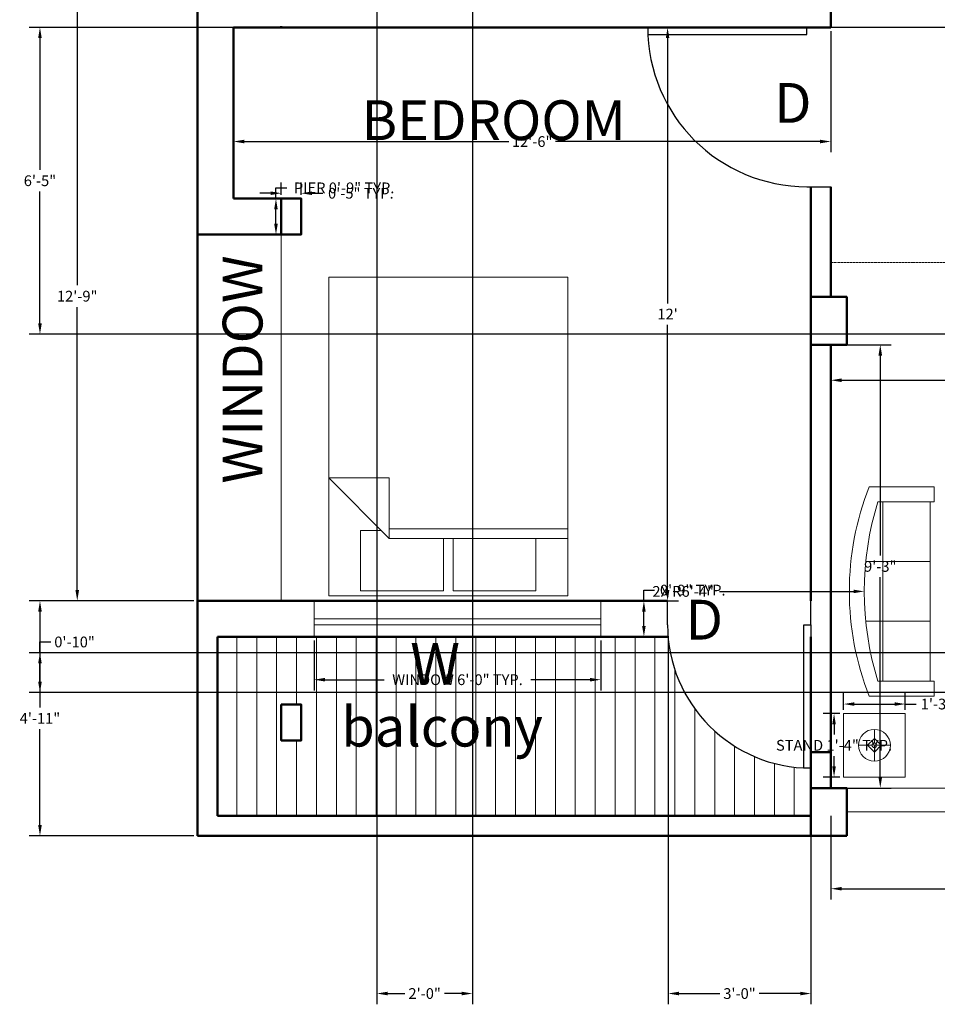
# Model space of a CAD drawing. Units: inches. Extents: x -15 to 796, y 111 to 651.
# Tile 1 of 6: x -15 to 216, y 126 to 373. Entities that reach past the tile are written whole.
import ezdxf

# ---------------------------------------------------------------- set-up
doc = ezdxf.new("R2010")
doc.units = ezdxf.units.IN
doc.header["$MEASUREMENT"] = 0
doc.linetypes.add('DASHED2', pattern=[0.375, 0.25, -0.125])
doc.layers.get('0').update_dxf_attribs({"color": 1})
for name, color, linetype, lineweight in [('A-ANNO-DIMS', 2, 'Continuous', 18), ('A-ANNO-TEXT', 7, 'Continuous', 18), ('A-AREA-IDEN', 7, 'Continuous', 25), ('A-COLS', 1, 'Continuous', 50), ('A-DOOR', 3, 'Continuous', 25), ('A-FLOR-PATT', 18, 'Continuous', 13), ('A-FURN', 8, 'Continuous', 18), ('A-GLAZ', 4, 'Continuous', 18), ('A-WALL', 7, 'Continuous', 50), ('A-WALL-OVHD', 7, 'DASHED2', 18)]:
    doc.layers.add(name, color=color, linetype=linetype, lineweight=lineweight)
doc.styles.get("Standard").update_dxf_attribs({"font": 'arial.ttf'})
doc.dimstyles.get("Standard").update_dxf_attribs({"dimscale": 15, "dimtxt": 0.18, "dimasz": 0.18, "dimexe": 0.18, "dimexo": 0.0625, "dimgap": 0.09, "dimtad": 0, "dimtih": 1, "dimtoh": 1, "dimdec": 0, "dimzin": 0, "dimdsep": 46, "dimlunit": 3, "dimtxsty": 'Standard', "dimcen": 0.09, "dimadec": 0, "dimazin": 0, "dimtfac": 1, "dimtdec": 0, "dimtofl": 0, "dimtmove": 0, "dimatfit": 3, "dimfxl": 1, "dimtolj": 1, "dimtzin": 0, "dimarcsym": 0})

# ---------------------------------------------------------------- blocks, each defined once
blk = doc.blocks.new('*U2')
for p, q in [((-36, 0), (-36, 6)), ((0, 0), (0, 6))]:
    blk.add_line(p, q)
blk.add_lwpolyline([(0, 0), (0, -36), (-1.75, -36), (-1.75, 0)], close=True)
blk.add_arc((0, 0), 36, 180, 270)
blk = doc.blocks.new('Bed - Queen')
for p, q in [((0, -80.00003), (0, 0)), ((0, 0), (59.99999, 0)), ((59.99999, 0), (59.99999, -80.00003)), ((7.99999, -1.2), (28.79998, -1.2)), ((7.99999, -14.4), (7.99999, -1.2)), ((28.79998, -1.2), (28.79998, -14.4)), ((31.19999, -1.2), (51.99999, -1.2)), ((31.19999, -14.4), (31.19999, -1.2)), ((51.99999, -1.2), (51.99999, -16.4)), ((0, -14.4), (44.8, -14.4)), ((59.99999, -29.6), (44.8, -14.4)), ((44.8, -14.4), (44.8, -29.6)), ((44.8, -16.8), (0, -16.8)), ((51.99999, -16.4), (46.79936, -16.4)), ((44.8, -29.6), (59.99999, -29.6)), ((59.99999, -80.00003), (0, -80.00003))]:
    blk.add_line(p, q)
blk = doc.blocks.new('*U4')
for p, q in [((0, 0), (0, -6)), ((-40, 0), (-40, -6))]:
    blk.add_line(p, q)
blk.add_lwpolyline([(0, 0), (0, 40), (-1.75, 40), (-1.75, 0)], close=True)
blk.add_arc((0, 0), 40, 90, 180)
blk = doc.blocks.new('Lamp - Table')
for p, q in [((0, 7), (0, 1)), ((-1, 0), (-7, 0)), ((0, 3), (-3, 0)), ((-3, 0), (0, -3)), ((3, 0), (0, 3)), ((0, -3), (3, 0)), ((1, 0), (7, 0)), ((0, -1), (0, -7))]:
    blk.add_line(p, q)
for radius in [7, 1]:
    blk.add_circle((0, 0), radius)
blk = doc.blocks.new('Sofa - Roundback 7 ft.')
for p, q in [((-12.00002, -32.4421), (-12.00003, -6.5971)), ((11.99997, -32.4421), (11.99998, -6.5971)), ((-36.000027, -34), (-36.000027, -11.4696)), ((35.99998, -34), (35.99998, -11.4696)), ((-35.999844, -13.3819), (35.9998, -13.3819)), ((-36.000027, -32.4421), (35.99998, -32.4421))]:
    blk.add_line(p, q)
for points in [[(-36.000027, -34), (-42.000027, -34), (-42.000027, -8)], [(41.99998, -8), (41.99998, -34), (35.99998, -34)]]:
    blk.add_lwpolyline(points)
for centre, radius, start, end in [((0, -114.25), 114.25, 68.43141, 111.5686), ((-0.00001, -127.1968), 121.1968, 72.72033, 107.2797)]:
    blk.add_arc(centre, radius, start, end)
blk = doc.blocks.new('*D19')
at = {"layer": 'A-ANNO-DIMS', "color": 0, "lineweight": -2, "transparency": 16777216}
for p, q in [((29.24, 380.13), (-2.76, 380.13)), ((-0.06, 377.43), (-0.06, 306.36)), ((-0.06, 229.83), (-0.06, 300.9)), ((29.24, 227.13), (-2.76, 227.13))]:
    blk.add_line(p, q, dxfattribs=at)
at = {"layer": 'A-ANNO-DIMS', "color": 0, "transparency": 16777216}
for points in [[(-0.51, 377.43), (0.39, 377.43), (-0.06, 380.13)], [(-0.51, 229.83), (0.39, 229.83), (-0.06, 227.13)]]:
    blk.add_solid(points, dxfattribs=at)
at = {"layer": 'Defpoints', "color": 0, "transparency": 16777216}
for p in [(30.18, 380.13), (-0.06, 227.13), (30.18, 227.13)]:
    blk.add_point(p, dxfattribs=at)
at = {"layer": 'A-ANNO-DIMS', "color": 0, "transparency": 16777216, "insert": (-0.06, 303.63), "char_height": 2.7, "attachment_point": 5}
blk.add_mtext('\\A1;12\'-9"', dxfattribs=at)
blk = doc.blocks.new('*D20')
at = {"layer": 'A-ANNO-DIMS', "color": 0, "lineweight": -2, "transparency": 16777216}
for p, q in [((39.18, 370.19), (39.18, 339.76)), ((189.18, 370.19), (189.18, 339.76)), ((41.88, 342.46), (108.32, 342.46)), ((186.48, 342.46), (120.04, 342.46))]:
    blk.add_line(p, q, dxfattribs=at)
at = {"layer": 'A-ANNO-DIMS', "color": 0, "transparency": 16777216}
for points in [[(41.88, 342.91), (41.88, 342.01), (39.18, 342.46)], [(186.48, 342.91), (186.48, 342.01), (189.18, 342.46)]]:
    blk.add_solid(points, dxfattribs=at)
at = {"layer": 'Defpoints', "color": 0, "transparency": 16777216}
for p in [(39.18, 371.13), (189.18, 371.13), (39.18, 342.46)]:
    blk.add_point(p, dxfattribs=at)
at = {"layer": 'A-ANNO-DIMS', "color": 0, "transparency": 16777216, "insert": (114.18, 342.46), "char_height": 2.7, "attachment_point": 5}
blk.add_mtext('\\A1;12\'-6"', dxfattribs=at)
blk = doc.blocks.new('*D21')
at = {"layer": 'A-ANNO-DIMS', "color": 0, "lineweight": -2, "transparency": 16777216}
for p, q in [((190.12, 291.43), (204.29, 291.43)), ((201.59, 288.73), (201.59, 238.51)), ((201.59, 182.83), (201.59, 233.05)), ((190.12, 180.13), (204.29, 180.13))]:
    blk.add_line(p, q, dxfattribs=at)
at = {"layer": 'A-ANNO-DIMS', "color": 0, "transparency": 16777216}
for points in [[(201.14, 288.73), (202.04, 288.73), (201.59, 291.43)], [(201.14, 182.83), (202.04, 182.83), (201.59, 180.13)]]:
    blk.add_solid(points, dxfattribs=at)
at = {"layer": 'Defpoints', "color": 0, "transparency": 16777216}
for p in [(189.18, 291.43), (189.18, 180.13), (201.59, 180.13)]:
    blk.add_point(p, dxfattribs=at)
at = {"layer": 'A-ANNO-DIMS', "color": 0, "transparency": 16777216, "insert": (201.59, 235.78), "char_height": 2.7, "attachment_point": 5}
blk.add_mtext('\\A1;9\'-3"', dxfattribs=at)
blk = doc.blocks.new('*D26')
at = {"layer": 'A-ANNO-DIMS', "color": 0, "lineweight": -2, "transparency": 16777216}
for p, q in [((133.96, 371.13), (150.88, 371.13)), ((148.18, 368.43), (148.18, 301.83)), ((148.18, 229.83), (148.18, 296.42)), ((133.96, 227.13), (150.88, 227.13))]:
    blk.add_line(p, q, dxfattribs=at)
at = {"layer": 'A-ANNO-DIMS', "color": 0, "transparency": 16777216}
for points in [[(147.73, 368.43), (148.63, 368.43), (148.18, 371.13)], [(147.73, 229.83), (148.63, 229.83), (148.18, 227.13)]]:
    blk.add_solid(points, dxfattribs=at)
at = {"layer": 'Defpoints', "color": 0, "transparency": 16777216}
for p in [(133.02, 371.13), (133.02, 227.13), (148.18, 227.13)]:
    blk.add_point(p, dxfattribs=at)
at = {"layer": 'A-ANNO-DIMS', "color": 0, "transparency": 16777216, "insert": (148.18, 299.13), "char_height": 2.7, "attachment_point": 5}
blk.add_mtext("\\A1;12'", dxfattribs=at)
blk = doc.blocks.new('*D27')
at = {"layer": 'A-ANNO-DIMS', "color": 0, "lineweight": -2, "transparency": 16777216}
for p, q in [((189.18, 283.46), (189.18, 285.22)), ((311.36, 284.98), (311.36, 279.82)), ((191.88, 282.52), (244.41, 282.52)), ((308.66, 282.52), (256.13, 282.52))]:
    blk.add_line(p, q, dxfattribs=at)
at = {"layer": 'A-ANNO-DIMS', "color": 0, "transparency": 16777216}
for points in [[(191.88, 282.97), (191.88, 282.07), (189.18, 282.52)], [(308.66, 282.97), (308.66, 282.07), (311.36, 282.52)]]:
    blk.add_solid(points, dxfattribs=at)
at = {"layer": 'Defpoints', "color": 0, "transparency": 16777216}
for p in [(311.36, 285.92), (189.18, 282.52), (189.18, 282.52)]:
    blk.add_point(p, dxfattribs=at)
at = {"layer": 'A-ANNO-DIMS', "color": 0, "transparency": 16777216, "insert": (250.27, 282.52), "char_height": 2.7, "attachment_point": 5}
blk.add_mtext('\\A1;10\'-2"', dxfattribs=at)
blk = doc.blocks.new('WIN-BEDROOM-72IN')
for p, q in [((0, 4.5), (72, 4.5)), ((0, 2.96), (72, 2.96))]:
    blk.add_line(p, q)
blk.add_lwpolyline([(0, 9), (72, 9), (72, 0), (0, 0)], close=True)
blk = doc.blocks.new('WIN-LIVING-PAIRED')
for p, q in [((62.78, 7.78), (65.45, 7.78)), ((62.78, 0), (62.78, 7.78)), ((65.45, 7.78), (65.45, 0)), ((0, 6), (62.78, 6)), ((65.45, 6), (128.5, 6)), ((4, 0), (124, 0)), ((65.45, 0), (62.78, 0))]:
    blk.add_line(p, q)
blk = doc.blocks.new('COL-9X12')
blk.add_lwpolyline([(9, 0), (0, 0), (0, 12), (9, 12)], close=True)
blk = doc.blocks.new('PIER-5X9')
blk.add_lwpolyline([(0, 9), (5, 9), (5, 0), (0, 0)], close=True)
blk = doc.blocks.new('TABLE-LAMP-STAND')
blk.add_lwpolyline([(0, 0), (15.51, 0), (15.51, 15.93), (0, 15.93)], close=True)
blk = doc.blocks.new('*D37')
at = {"layer": 'A-ANNO-DIMS', "color": 0, "lineweight": -2, "transparency": 16777216}
for p, q in [((49.84, 328.13), (49.84, 330.83)), ((49.84, 330.83), (52.54, 330.83)), ((50.25, 328.13), (47.14, 328.13)), ((49.84, 321.83), (49.84, 325.43)), ((50.25, 319.13), (47.14, 319.13))]:
    blk.add_line(p, q, dxfattribs=at)
at = {"layer": 'A-ANNO-DIMS', "color": 0, "transparency": 16777216}
for points in [[(49.39, 325.43), (50.29, 325.43), (49.84, 328.13)], [(49.39, 321.83), (50.29, 321.83), (49.84, 319.13)]]:
    blk.add_solid(points, dxfattribs=at)
at = {"layer": 'Defpoints', "color": 0, "transparency": 16777216}
for p in [(49.84, 328.13), (51.19, 328.13), (51.19, 319.13)]:
    blk.add_point(p, dxfattribs=at)
at = {"layer": 'A-ANNO-DIMS', "color": 0, "transparency": 16777216, "insert": (66.97, 330.83), "char_height": 2.7, "attachment_point": 5}
blk.add_mtext('\\A1;PIER 0\'-9" TYP.', dxfattribs=at)
blk = doc.blocks.new('*D38')
at = {"layer": 'A-ANNO-DIMS', "color": 0, "lineweight": -2, "transparency": 16777216}
for p, q in [((51.19, 329.06), (51.19, 332.18)), ((56.19, 329.06), (56.19, 332.18)), ((48.49, 329.48), (45.79, 329.48)), ((58.89, 329.48), (61.59, 329.48))]:
    blk.add_line(p, q, dxfattribs=at)
at = {"layer": 'A-ANNO-DIMS', "color": 0, "transparency": 16777216}
for points in [[(48.49, 329.93), (48.49, 329.03), (51.19, 329.48)], [(58.89, 329.93), (58.89, 329.03), (56.19, 329.48)]]:
    blk.add_solid(points, dxfattribs=at)
at = {"layer": 'Defpoints', "color": 0, "transparency": 16777216}
for p in [(56.19, 329.48), (51.19, 328.13), (56.19, 328.13)]:
    blk.add_point(p, dxfattribs=at)
at = {"layer": 'A-ANNO-DIMS', "color": 0, "transparency": 16777216, "insert": (71.16, 329.48), "char_height": 2.7, "attachment_point": 5}
blk.add_mtext('\\A1;0\'-5" TYP.', dxfattribs=at)
blk = doc.blocks.new('*D59')
at = {"layer": 'A-ANNO-DIMS', "color": 0, "lineweight": -2, "transparency": 16777216}
for p, q in [((59.43, 217.19), (59.43, 204.63)), ((131.43, 217.19), (131.43, 204.63)), ((62.13, 207.33), (77, 207.33)), ((128.73, 207.33), (113.86, 207.33))]:
    blk.add_line(p, q, dxfattribs=at)
at = {"layer": 'A-ANNO-DIMS', "color": 0, "transparency": 16777216}
for points in [[(62.13, 207.78), (62.13, 206.88), (59.43, 207.33)], [(128.73, 207.78), (128.73, 206.88), (131.43, 207.33)]]:
    blk.add_solid(points, dxfattribs=at)
at = {"layer": 'Defpoints', "color": 0, "transparency": 16777216}
for p in [(59.43, 218.13), (131.43, 218.13), (131.43, 207.33)]:
    blk.add_point(p, dxfattribs=at)
at = {"layer": 'A-ANNO-DIMS', "color": 0, "transparency": 16777216, "insert": (95.43, 207.33), "char_height": 2.7, "attachment_point": 5}
blk.add_mtext('\\A1;WINDOW 6\'-0" TYP.', dxfattribs=at)
blk = doc.blocks.new('*D60')
at = {"layer": 'A-ANNO-DIMS', "color": 0, "lineweight": -2, "transparency": 16777216}
for p, q in [((142.23, 227.13), (142.23, 229.83)), ((142.23, 229.83), (144.93, 229.83)), ((132.37, 227.13), (144.93, 227.13)), ((142.23, 220.83), (142.23, 224.43)), ((132.37, 218.13), (144.93, 218.13))]:
    blk.add_line(p, q, dxfattribs=at)
at = {"layer": 'A-ANNO-DIMS', "color": 0, "transparency": 16777216}
for points in [[(141.78, 224.43), (142.68, 224.43), (142.23, 227.13)], [(141.78, 220.83), (142.68, 220.83), (142.23, 218.13)]]:
    blk.add_solid(points, dxfattribs=at)
at = {"layer": 'Defpoints', "color": 0, "transparency": 16777216}
for p in [(131.43, 227.13), (142.23, 227.13), (131.43, 218.13)]:
    blk.add_point(p, dxfattribs=at)
at = {"layer": 'A-ANNO-DIMS', "color": 0, "transparency": 16777216, "insert": (154.51, 229.83), "char_height": 2.7, "attachment_point": 5}
blk.add_mtext('\\A1;0\'-9" TYP.', dxfattribs=at)
blk = doc.blocks.new('*D63')
at = {"layer": 'A-ANNO-DIMS', "color": 0, "lineweight": -2, "transparency": 16777216}
for p, q in [((189.18, 173.19), (189.18, 152.15)), ((317.68, 173.19), (317.68, 152.15)), ((191.88, 154.85), (223.38, 154.85)), ((314.98, 154.85), (283.48, 154.85))]:
    blk.add_line(p, q, dxfattribs=at)
at = {"layer": 'A-ANNO-DIMS', "color": 0, "transparency": 16777216}
for points in [[(191.88, 155.3), (191.88, 154.4), (189.18, 154.85)], [(314.98, 155.3), (314.98, 154.4), (317.68, 154.85)]]:
    blk.add_solid(points, dxfattribs=at)
at = {"layer": 'Defpoints', "color": 0, "transparency": 16777216}
for p in [(189.18, 174.13), (317.68, 174.13), (317.68, 154.85)]:
    blk.add_point(p, dxfattribs=at)
at = {"layer": 'A-ANNO-DIMS', "color": 0, "transparency": 16777216, "insert": (253.43, 154.85), "char_height": 2.7, "attachment_point": 5}
blk.add_mtext('\\A1;PAIRED WINDOW 10\'-8 1/2" TYP.', dxfattribs=at)
blk = doc.blocks.new('*D65')
at = {"layer": 'A-ANNO-DIMS', "color": 0, "lineweight": -2, "transparency": 16777216}
for p, q in [((191.43, 198.83), (187.28, 198.83)), ((189.98, 196.13), (189.98, 193.61)), ((189.98, 185.6), (189.98, 188.12)), ((191.43, 182.9), (187.28, 182.9))]:
    blk.add_line(p, q, dxfattribs=at)
at = {"layer": 'A-ANNO-DIMS', "color": 0, "transparency": 16777216}
for points in [[(189.53, 196.13), (190.43, 196.13), (189.98, 198.83)], [(189.53, 185.6), (190.43, 185.6), (189.98, 182.9)]]:
    blk.add_solid(points, dxfattribs=at)
at = {"layer": 'Defpoints', "color": 0, "transparency": 16777216}
for p in [(189.98, 198.83), (192.37, 198.83), (192.37, 182.9)]:
    blk.add_point(p, dxfattribs=at)
at = {"layer": 'A-ANNO-DIMS', "color": 0, "transparency": 16777216, "insert": (189.98, 190.86), "char_height": 2.7, "attachment_point": 5}
blk.add_mtext('\\A1;STAND 1\'-4" TYP.', dxfattribs=at)
blk = doc.blocks.new('*D66')
at = {"layer": 'A-ANNO-DIMS', "color": 0, "lineweight": -2, "transparency": 16777216}
for p, q in [((192.37, 199.77), (192.37, 203.92)), ((207.87, 199.77), (207.87, 203.92)), ((195.07, 201.22), (205.17, 201.22)), ((207.87, 201.22), (210.57, 201.22))]:
    blk.add_line(p, q, dxfattribs=at)
at = {"layer": 'A-ANNO-DIMS', "color": 0, "transparency": 16777216}
for points in [[(195.07, 201.67), (195.07, 200.77), (192.37, 201.22)], [(205.17, 201.67), (205.17, 200.77), (207.87, 201.22)]]:
    blk.add_solid(points, dxfattribs=at)
at = {"layer": 'Defpoints', "color": 0, "transparency": 16777216}
for p in [(207.87, 201.22), (192.37, 198.83), (207.87, 198.83)]:
    blk.add_point(p, dxfattribs=at)
at = {"layer": 'A-ANNO-DIMS', "color": 0, "transparency": 16777216, "insert": (223.17, 201.22), "char_height": 2.7, "attachment_point": 5}
blk.add_mtext('\\A1;1\'-3 1/2" TYP.', dxfattribs=at)
blk = doc.blocks.new('*D69')
at = {"layer": 'A-ANNO-DIMS', "color": 0, "lineweight": -2, "transparency": 16777216}
for p, q in [((-9.42, 214.11), (-9.42, 216.81)), ((-9.42, 216.81), (-6.72, 216.81)), ((408.74, 214.11), (-12.12, 214.11)), ((-9.42, 206.81), (-9.42, 211.41)), ((408.74, 204.11), (-12.12, 204.11))]:
    blk.add_line(p, q, dxfattribs=at)
at = {"layer": 'A-ANNO-DIMS', "color": 0, "transparency": 16777216}
for points in [[(-9.87, 211.41), (-8.97, 211.41), (-9.42, 214.11)], [(-9.87, 206.81), (-8.97, 206.81), (-9.42, 204.11)]]:
    blk.add_solid(points, dxfattribs=at)
at = {"layer": 'Defpoints', "color": 0, "transparency": 16777216}
for p in [(-9.42, 214.11), (409.68, 214.11), (409.68, 204.11)]:
    blk.add_point(p, dxfattribs=at)
at = {"layer": 'A-ANNO-DIMS', "color": 0, "transparency": 16777216, "insert": (-0.73, 216.81), "char_height": 2.7, "attachment_point": 5}
blk.add_mtext('\\A1;0\'-10"', dxfattribs=at)
blk = doc.blocks.new('*D72')
at = {"layer": 'A-ANNO-DIMS', "color": 0, "lineweight": -2, "transparency": 16777216}
for p, q in [((29.24, 227.13), (-12.12, 227.13)), ((-9.42, 224.43), (-9.42, 200.33)), ((-9.42, 170.83), (-9.42, 194.92)), ((29.24, 168.13), (-12.12, 168.13))]:
    blk.add_line(p, q, dxfattribs=at)
at = {"layer": 'A-ANNO-DIMS', "color": 0, "transparency": 16777216}
for points in [[(-9.87, 224.43), (-8.97, 224.43), (-9.42, 227.13)], [(-9.87, 170.83), (-8.97, 170.83), (-9.42, 168.13)]]:
    blk.add_solid(points, dxfattribs=at)
at = {"layer": 'Defpoints', "color": 0, "transparency": 16777216}
for p in [(-9.42, 227.13), (30.18, 227.13), (30.18, 168.13)]:
    blk.add_point(p, dxfattribs=at)
at = {"layer": 'A-ANNO-DIMS', "color": 0, "transparency": 16777216, "insert": (-9.42, 197.63), "char_height": 2.7, "attachment_point": 5}
blk.add_mtext('\\A1;4\'-11"', dxfattribs=at)
blk = doc.blocks.new('*D74')
at = {"layer": 'A-ANNO-DIMS', "color": 0, "lineweight": -2, "transparency": 16777216}
for p, q in [((413.24, 371.13), (-12.12, 371.13)), ((-9.42, 368.43), (-9.42, 335.35)), ((-9.42, 296.81), (-9.42, 329.89)), ((364.97, 294.11), (-12.12, 294.11))]:
    blk.add_line(p, q, dxfattribs=at)
at = {"layer": 'A-ANNO-DIMS', "color": 0, "transparency": 16777216}
for points in [[(-9.87, 368.43), (-8.97, 368.43), (-9.42, 371.13)], [(-9.87, 296.81), (-8.97, 296.81), (-9.42, 294.11)]]:
    blk.add_solid(points, dxfattribs=at)
at = {"layer": 'Defpoints', "color": 0, "transparency": 16777216}
for p in [(414.18, 371.13), (-9.42, 294.11), (365.91, 294.11)]:
    blk.add_point(p, dxfattribs=at)
at = {"layer": 'A-ANNO-DIMS', "color": 0, "transparency": 16777216, "insert": (-9.42, 332.62), "char_height": 2.7, "attachment_point": 5}
blk.add_mtext('\\A1;6\'-5"', dxfattribs=at)
blk = doc.blocks.new('*D79')
at = {"layer": 'A-ANNO-DIMS', "color": 0, "lineweight": -2, "transparency": 16777216}
for p, q in [((148.31, 217.19), (148.31, 125.83)), ((184.18, 184.19), (184.18, 125.83)), ((151.01, 128.53), (161.31, 128.53)), ((181.48, 128.53), (171.18, 128.53))]:
    blk.add_line(p, q, dxfattribs=at)
at = {"layer": 'A-ANNO-DIMS', "color": 0, "transparency": 16777216}
for points in [[(151.01, 128.98), (151.01, 128.08), (148.31, 128.53)], [(181.48, 128.98), (181.48, 128.08), (184.18, 128.53)]]:
    blk.add_solid(points, dxfattribs=at)
at = {"layer": 'Defpoints', "color": 0, "transparency": 16777216}
for p in [(148.31, 218.13), (184.18, 185.13), (184.18, 128.53)]:
    blk.add_point(p, dxfattribs=at)
at = {"layer": 'A-ANNO-DIMS', "color": 0, "transparency": 16777216, "insert": (166.24, 128.53), "char_height": 2.7, "attachment_point": 5}
blk.add_mtext('\\A1;3\'-0"', dxfattribs=at)
blk = doc.blocks.new('*D80')
at = {"layer": 'A-ANNO-DIMS', "color": 0, "lineweight": -2, "transparency": 16777216}
for p, q in [((75.18, 528.19), (75.18, 125.83)), ((99.18, 527.44), (99.18, 125.83)), ((77.88, 128.53), (82.22, 128.53)), ((96.48, 128.53), (92.14, 128.53))]:
    blk.add_line(p, q, dxfattribs=at)
at = {"layer": 'A-ANNO-DIMS', "color": 0, "transparency": 16777216}
for points in [[(77.88, 128.98), (77.88, 128.08), (75.18, 128.53)], [(96.48, 128.98), (96.48, 128.08), (99.18, 128.53)]]:
    blk.add_solid(points, dxfattribs=at)
at = {"layer": 'Defpoints', "color": 0, "transparency": 16777216}
for p in [(75.18, 529.13), (99.18, 528.38), (75.18, 128.53)]:
    blk.add_point(p, dxfattribs=at)
at = {"layer": 'A-ANNO-DIMS', "color": 0, "transparency": 16777216, "insert": (87.18, 128.53), "char_height": 2.7, "attachment_point": 5}
blk.add_mtext('\\A1;2\'-0"', dxfattribs=at)
blk = doc.blocks.new('*D84')
at = {"layer": 'A-ANNO-DIMS', "color": 0, "lineweight": -2, "transparency": 16777216}
for p, q in [((273.39, 228.15), (273.39, 230.85)), ((161.25, 229.5), (194.88, 229.5)), ((272.04, 229.5), (274.74, 229.5))]:
    blk.add_line(p, q, dxfattribs=at)
at = {"layer": 'A-ANNO-DIMS', "color": 0, "transparency": 16777216}
blk.add_solid([(194.88, 229.95), (194.88, 229.05), (197.58, 229.5)], dxfattribs=at)
at = {"layer": 'Defpoints', "color": 0, "transparency": 16777216}
for p in [(197.58, 229.5), (273.39, 229.5)]:
    blk.add_point(p, dxfattribs=at)
at = {"layer": 'A-ANNO-DIMS', "color": 0, "transparency": 16777216, "insert": (152.09, 229.5), "char_height": 2.7, "attachment_point": 5}
blk.add_mtext('\\A1;2X R6\'-4"', dxfattribs=at)

msp = doc.modelspace()

# ---------------------------------------------------------------- hatches: boundary and pattern name
at = {"layer": 'A-FLOR-PATT'}
h = msp.add_hatch(dxfattribs=at)
h.set_pattern_fill('_USER', color=256, scale=5, angle=90, pattern_type=0)
h.set_pattern_definition([(90, (0, 0), (-5, 3e-16), [])])
h.paths.add_polyline_path([(35.18, 218.13), (35.18, 173.13), (184.18, 173.13), (184.18, 185.13), (182.43, 185.13), (182.43, 185.17, -0.376042), (148.31, 218.13)])
h.paths.add_polyline_path([(56.19, 192.09), (51.19, 192.09), (51.19, 201.09), (56.19, 201.09)], flags=16)

# ---------------------------------------------------------------- linework, layer by layer
at = {"layer": 'A-GLAZ'}
msp.add_line((51.19, 328.13), (51.19, 227.43), dxfattribs=at)
at = {"layer": 'A-WALL'}
for p, q in [((30.18, 380.13), (30.18, 227.13)), ((189.18, 380.13), (189.18, 371.13)), ((39.18, 371.13), (39.18, 328.13)), ((189.18, 371.13), (39.18, 371.13)), ((51.19, 371.43), (51.19, 371.13)), ((184.18, 227.13), (184.18, 331.13)), ((189.18, 331.13), (189.18, 303.43)), ((39.18, 328.13), (51.19, 328.13)), ((30.18, 319.13), (51.19, 319.13)), ((189.18, 291.43), (189.18, 180.13)), ((30.18, 168.13), (30.18, 227.13)), ((30.18, 227.13), (148.18, 227.13)), ((30.18, 227.13), (148.18, 227.13)), ((35.18, 218.13), (148.31, 218.13)), ((35.18, 173.13), (35.18, 218.13)), ((184.18, 218.13), (184.18, 173.13)), ((184.18, 173.13), (35.18, 173.13)), ((193.18, 168.13), (30.18, 168.13))]:
    msp.add_line(p, q, dxfattribs=at)
at = {"layer": 'A-WALL-OVHD'}
msp.add_line((253.43, 312.13), (189.18, 312.13), dxfattribs=at)

# ---------------------------------------------------------------- block references
at = {"layer": 'A-COLS'}
for name, p in [('PIER-5X9', (51.19, 319.13)), ('PIER-5X9', (51.19, 192.09)), ('PIER-5X9', (184.17, 180.13)), ('COL-9X12', (184.18, 168.13))]:
    msp.add_blockref(name, p, dxfattribs=at)
at = {"layer": 'A-COLS', "rotation": 180}
msp.add_blockref('COL-9X12', (193.18, 303.43), dxfattribs=at)
at = {"layer": 'A-DOOR', "rotation": 90}
msp.add_blockref('*U4', (183.18, 371.13), dxfattribs=at)
at = {"layer": 'A-DOOR'}
msp.add_blockref('*U2', (184.18, 221.13), dxfattribs=at)
at = {"layer": 'A-FURN', "rotation": 180}
msp.add_blockref('Bed - Queen', (123.11, 228.42), dxfattribs=at)
at = {"layer": 'A-FURN', "xscale": 0.6255113727593298, "yscale": 0.6255113727593298, "zscale": 0.6255113727593298, "rotation": 90}
msp.add_blockref('Sofa - Roundback 7 ft.', (193.82, 229.5), dxfattribs=at)
at = {"layer": 'A-FURN'}
msp.add_blockref('TABLE-LAMP-STAND', (192.37, 182.9), dxfattribs=at)
at = {"layer": 'A-FURN', "xscale": 0.5714285204081744, "yscale": 0.5714285204081744, "zscale": 0.5714285204081744}
msp.add_blockref('Lamp - Table', (200.12, 190.86), dxfattribs=at)
at = {"layer": 'A-GLAZ'}
for name, p in [('WIN-BEDROOM-72IN', (59.43, 218.13)), ('WIN-LIVING-PAIRED', (189.18, 174.13))]:
    msp.add_blockref(name, p, dxfattribs=at)

# ---------------------------------------------------------------- texts
at = {"layer": 'A-ANNO-TEXT'}
msp.add_text('WINDOW', height=10, rotation=90, dxfattribs=at).set_placement((46.46, 256.56))
at = {"layer": 'A-ANNO-TEXT', "attachment_point": 1}
for s, width, gutter_width, insert, char_height in [('D', 13.2435, 1, (174.93, 357.16), 10), ('D', 13.2435, 1, (152.72, 227.4), 10), ('W', 19.9719, 52.27, (83.55, 216.52), 10.45)]:
    msp.add_mtext_dynamic_manual_height_columns(s, width=width, gutter_width=gutter_width, heights=[0], dxfattribs=dict(at, insert=insert, char_height=char_height))
at = {"layer": 'A-AREA-IDEN', "char_height": 10, "attachment_point": 1}
for s, width, gutter_width, insert in [('BEDROOM', 27.6124, 50, (71.31, 352.81)), ('balcony', 26.4166, 1, (66.22, 200.55))]:
    msp.add_mtext_dynamic_manual_height_columns(s, width=width, gutter_width=gutter_width, heights=[0], dxfattribs=dict(at, insert=insert))

# ---------------------------------------------------------------- dimensions: what is measured, and where the dimension line sits
at = {"layer": 'A-ANNO-DIMS'}
for base, p1, p2, override, picture, middle in [((75.18, 128.53), (99.18, 528.38), (75.18, 529.13), {"dimdec": 1, "dimlfac": 1, "dimrnd": 0, "dimzin": 1, "dimdsep": 46, "dimlunit": 4, "dimfrac": 2}, '*D80', (87.18, 128.53)), ((39.18, 342.46), (189.18, 371.13), (39.18, 371.13), {"dimclrd": 0, "dimclre": 0, "dimclrt": 0}, '*D20', (114.18, 342.46)), ((189.18, 282.52), (311.36, 285.92), (189.18, 282.52), {"dimclrd": 0, "dimclre": 0, "dimclrt": 0}, '*D27', (250.27, 282.52)), ((184.18, 128.53), (148.31, 218.13), (184.18, 185.13), {"dimdec": 1, "dimlfac": 1, "dimrnd": 0, "dimzin": 1, "dimdsep": 46, "dimlunit": 4, "dimfrac": 2}, '*D79', (166.24, 128.53))]:
    dim = msp.add_linear_dim(base=base, p1=p1, p2=p2, dimstyle='Standard', override=override, dxfattribs=at)
    dim.commit()
    dim.dimension.update_dxf_attribs({"geometry": picture, "text_midpoint": middle})
for base, p1, p2, override, picture, middle in [((-0.06, 227.13), (30.18, 380.13), (30.18, 227.13), {"dimclrd": 0, "dimclre": 0, "dimclrt": 0}, '*D19', (-0.06, 303.63)), ((-9.42, 294.11), (414.18, 371.13), (365.91, 294.11), {"dimdec": 1, "dimlfac": 1, "dimrnd": 0, "dimzin": 1, "dimdsep": 46, "dimlunit": 4, "dimfrac": 2}, '*D74', (-9.42, 332.62)), ((148.18, 227.13), (133.02, 371.13), (133.02, 227.13), {"dimclrd": 0, "dimclre": 0, "dimclrt": 0}, '*D26', (148.18, 299.13)), ((201.59, 180.13), (189.18, 291.43), (189.18, 180.13), {"dimclrd": 0, "dimclre": 0, "dimclrt": 0}, '*D21', (201.59, 235.78)), ((-9.42, 227.13), (30.18, 168.13), (30.18, 227.13), {"dimdec": 1, "dimlfac": 1, "dimrnd": 0, "dimzin": 1, "dimdsep": 46, "dimlunit": 4, "dimfrac": 2}, '*D72', (-9.42, 197.63)), ((-9.42, 214.11), (409.68, 204.11), (409.68, 214.11), {"dimdec": 1, "dimlfac": 1, "dimrnd": 0, "dimzin": 1, "dimdsep": 46, "dimlunit": 4, "dimfrac": 2}, '*D69', (-0.73, 216.81))]:
    dim = msp.add_linear_dim(base=base, p1=p1, p2=p2, angle=90, dimstyle='Standard', override=override, dxfattribs=at)
    dim.commit()
    dim.dimension.update_dxf_attribs({"geometry": picture, "text_midpoint": middle})
for base, p1, p2, text, picture, middle in [((49.84, 328.13), (51.19, 319.13), (51.19, 328.13), 'PIER <> TYP.', '*D37', (66.97, 330.83)), ((142.23, 227.13), (131.43, 218.13), (131.43, 227.13), '<> TYP.', '*D60', (154.51, 229.83)), ((189.98, 198.83), (192.37, 182.9), (192.37, 198.83), 'STAND <> TYP.', '*D65', (189.98, 190.86))]:
    dim = msp.add_linear_dim(base=base, p1=p1, p2=p2, angle=90, text=text, dimstyle='Standard', override={"dimdec": 1, "dimlfac": 1, "dimrnd": 0, "dimzin": 1, "dimdsep": 46, "dimlunit": 4, "dimfrac": 2}, dxfattribs=at)
    dim.commit()
    dim.dimension.update_dxf_attribs({"geometry": picture, "text_midpoint": middle})
for base, p1, p2, text, picture, middle in [((56.19, 329.48), (51.19, 328.13), (56.19, 328.13), '<> TYP.', '*D38', (71.16, 329.48)), ((131.43, 207.33), (59.43, 218.13), (131.43, 218.13), 'WINDOW <> TYP.', '*D59', (95.43, 207.33)), ((207.87, 201.22), (192.37, 198.83), (207.87, 198.83), '<> TYP.', '*D66', (223.17, 201.22)), ((317.68, 154.85), (189.18, 174.13), (317.68, 174.13), 'PAIRED WINDOW <> TYP.', '*D63', (253.43, 154.85))]:
    dim = msp.add_linear_dim(base=base, p1=p1, p2=p2, text=text, dimstyle='Standard', override={"dimdec": 1, "dimlfac": 1, "dimrnd": 0, "dimzin": 1, "dimdsep": 46, "dimlunit": 4, "dimfrac": 2}, dxfattribs=at)
    dim.commit()
    dim.dimension.update_dxf_attribs({"geometry": picture, "text_midpoint": middle})
dim = msp.add_radius_dim(center=(273.39, 229.5), mpoint=(197.58, 229.5), text='2X <>', dimstyle='Standard', override={"dimdec": 1, "dimlfac": 1, "dimrnd": 0, "dimzin": 1, "dimdsep": 46, "dimlunit": 4, "dimfrac": 2}, dxfattribs=at)
dim.commit()
dim.dimension.update_dxf_attribs({"geometry": '*D84', "text_midpoint": (152.09, 229.5), "dimtype": 164})

doc.saveas('drawing.dxf')
